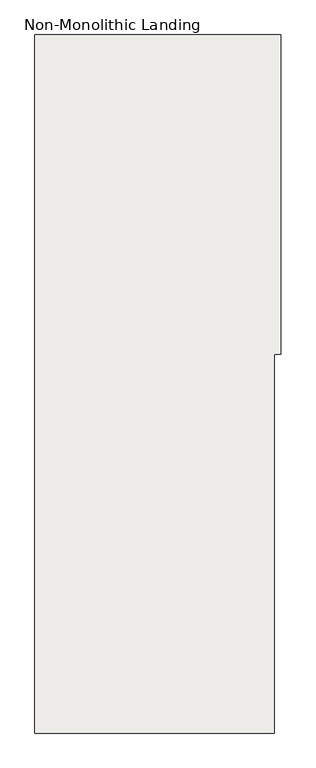
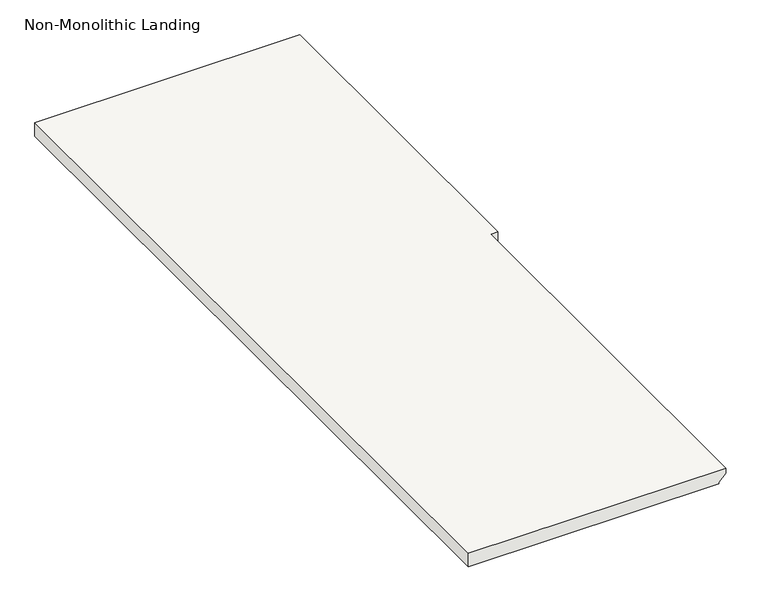
"""IFC4 building model written with IfcOpenShell, lengths in millimetres: slab geometry, Non-Monolithic Landing."""

from ifc_helpers import new_model, si_unit, origin, place, context, project, spatial, faceted_brep, source, transform, mapped, element, save


def non_monolithic_landing_6f104080(model_context):
    return source(origin(), model_context, "Body", "Brep", [
        faceted_brep([(-8123.4707895, 5014.1144188, 4781.55), (-8148.8707895, 5014.1144188, 4756.15), (-8148.8707895, 6233.3144188, 4756.15), (-8123.4707895, 6233.3144188, 4781.55), (-8123.4707895, 6461.9144188, 4800.6), (-8098.0707895, 6461.9144188, 4800.6), (-8098.0707895, 7681.1144188, 4800.6), (-8123.4707895, 7681.1144188, 4800.6), (-9037.8707895, 7681.1144188, 4800.6), (-9037.8707895, 5014.1144188, 4800.6), (-8123.4707895, 5014.1144188, 4800.6), (-8148.8707895, 6233.3144188, 4749.8), (-8148.8707895, 5014.1144188, 4749.8), (-9037.8707895, 5014.1144188, 4749.8), (-9037.8707895, 7681.1144188, 4749.8), (-8123.4707895, 7681.1144188, 4749.8), (-8098.0707895, 7681.1144188, 4749.8), (-8098.0707895, 6461.9144188, 4749.8), (-8123.4707895, 6461.9144188, 4749.8), (-8123.4707895, 6233.3144188, 4749.8)], [[[0, 1, 2, 3]], [[4, 5, 6, 7, 8, 9, 10]], [[11, 12, 13, 14, 15, 16, 17, 18, 19]], [[12, 11, 2, 1]], [[11, 19, 3, 2]], [[4, 10, 0, 3, 19, 18]], [[5, 4, 18, 17]], [[6, 5, 17, 16]], [[7, 6, 16, 15]], [[8, 7, 15, 14]], [[9, 8, 14, 13]], [[10, 9, 13, 12, 1, 0]]]),
    ])


if __name__ == "__main__":
    model = new_model("IFC4")
    model_context = context("Model", 3, world=origin())
    ifc_project = project(units=[si_unit("LENGTHUNIT", "METRE", prefix="MILLI")], contexts=[model_context])
    site = spatial("IfcSite", under=ifc_project)
    building = spatial("IfcBuilding", under=site)
    placement = place(None, origin())
    non_monolithic_landing_shape = non_monolithic_landing_6f104080(model_context)
    element("IfcSlab", 1, ObjectType="Non-Monolithic Landing", at=placement, inside=building, context=model_context, shape_type="MappedRepresentation", body=[
        mapped(non_monolithic_landing_shape, transform((0.0, 0.0, 0.0), x_axis=(1.0, 0.0, 0.0), y_axis=(0.0, 1.0, 0.0), z_axis=(0.0, 0.0, 1.0))),
    ])
    save(model, "model.ifc")
